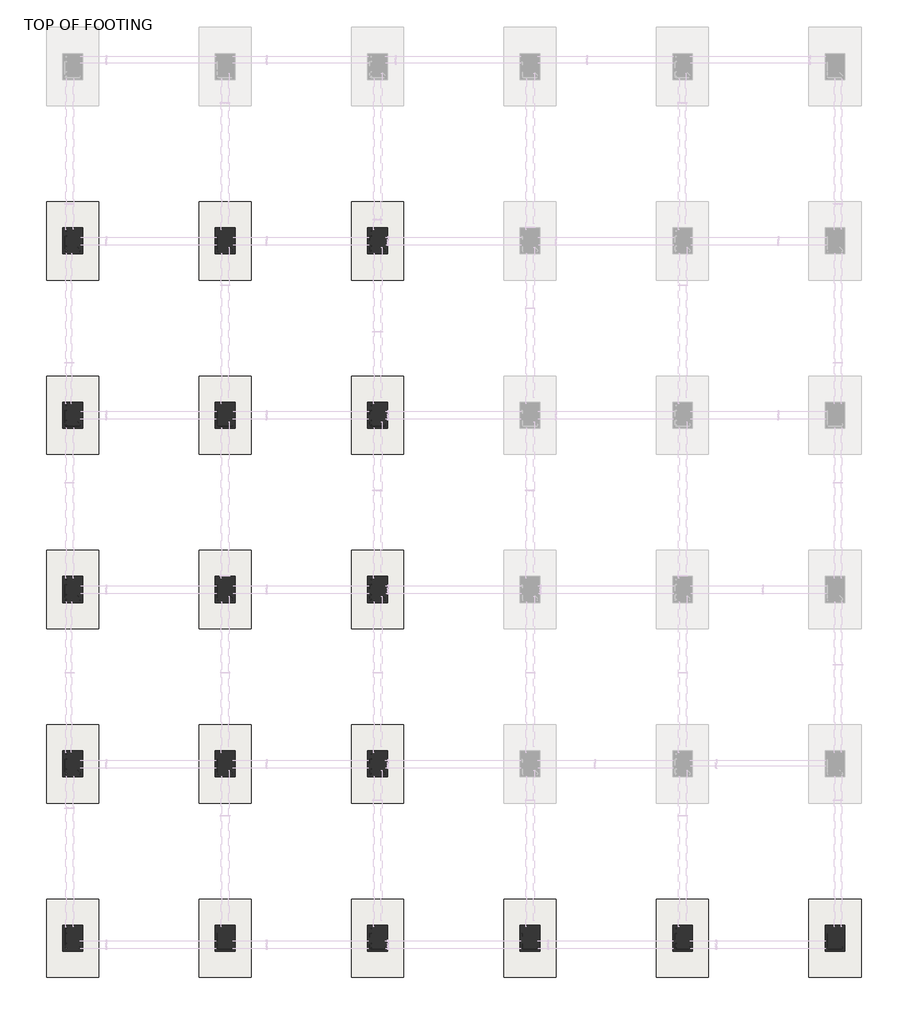
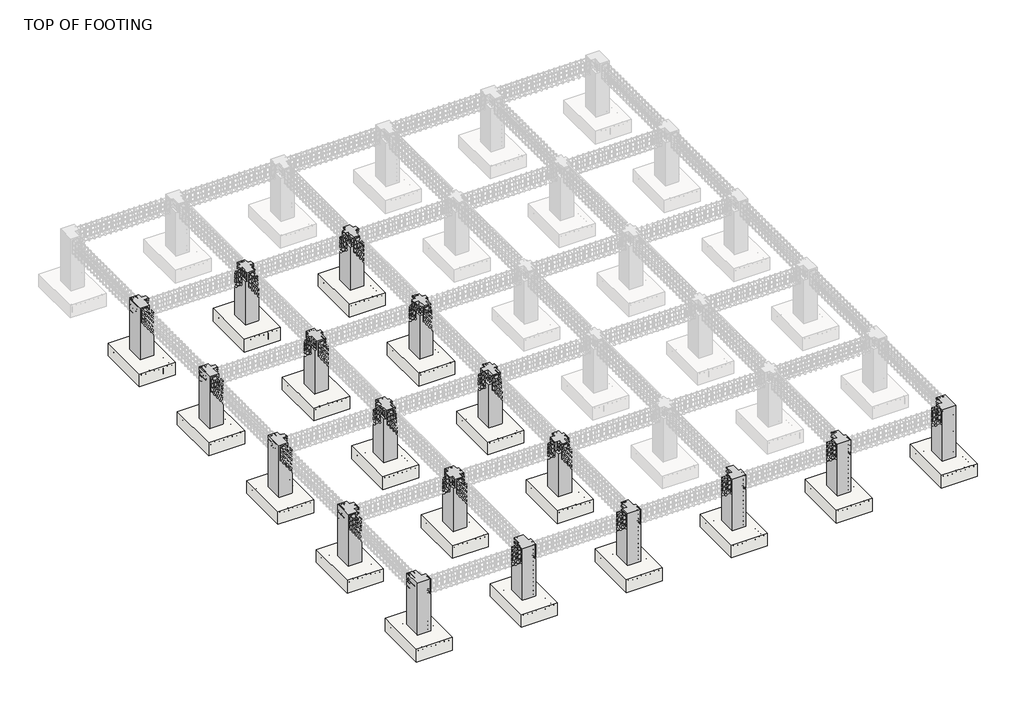
# One storey, part 1 of 33: 18 columns, 18 slabs.
"""IFC4 building model written with IfcOpenShell, lengths in millimetres."""

from ifc_helpers import new_model, si_unit, origin, place, context, project, spatial, faceted_brep, transform, mapped, element, save
from components import m_footing_rectangular_1800_x_1200_x_450mm_16ba7ea5

model = new_model("IFC4")

# Units and contexts
model_context = context("Model", 3, world=origin())
ifc_project = project(units=[si_unit("LENGTHUNIT", "METRE", prefix="MILLI")], contexts=[model_context])

# Site, building, storey
site = spatial("IfcSite", under=ifc_project)
building = spatial("IfcBuilding", under=site)
storey = spatial("IfcBuildingStorey", under=building, Name="TOP OF FOOTING", Elevation=-1828.8)

# Columns
placement = place(None, origin())
element("IfcColumn", 1, ObjectType="M_Concrete-Rectangular-Column : 450 x 600mm", at=placement, inside=storey, context=model_context, shape_type="Brep", body=[
    faceted_brep([(-8760.6788975, -214.4318674, -1828.8), (-8760.6788975, -814.4318674, -1828.8), (-9210.6788975, -814.4318674, -1828.8), (-9210.6788975, -214.4318674, -1828.8), (-8760.6788975, -214.4318674, -300.0), (-8760.6788975, -514.4318674, -300.0), (-8760.6788975, -514.4318674, 0.0), (-8760.6788975, -814.4318674, 0.0), (-9210.6788975, -814.4318674, 0.0), (-9210.6788975, -214.4318674, 0.0), (-8910.6788975, -214.4318674, 0.0), (-8910.6788975, -214.4318674, -300.0), (-8910.6788975, -514.4318674, 0.0), (-8910.6788975, -514.4318674, -300.0)], [[[0, 1, 2, 3]], [[1, 0, 4, 5, 6, 7]], [[2, 1, 7, 8]], [[3, 2, 8, 9]], [[0, 3, 9, 10, 11, 4]], [[8, 7, 6, 12, 10, 9]], [[11, 13, 5, 4]], [[13, 12, 6, 5]], [[12, 13, 11, 10]]]),
])
element("IfcColumn", 2, ObjectType="M_Concrete-Rectangular-Column : 450 x 600mm", at=placement, inside=storey, context=model_context, shape_type="Brep", body=[
    faceted_brep([(-8760.6788975, 3785.5681326, -1828.8), (-8760.6788975, 3185.5681326, -1828.8), (-9210.6788975, 3185.5681326, -1828.8), (-9210.6788975, 3785.5681326, -1828.8), (-8760.6788975, 3785.5681326, -300.0), (-8760.6788975, 3635.5681326, -300.0), (-8760.6788975, 3635.5681326, 0.0), (-8760.6788975, 3335.5681326, 0.0), (-8760.6788975, 3335.5681326, -300.0), (-8760.6788975, 3185.5681326, -300.0), (-8910.6788975, 3185.5681326, -300.0), (-8910.6788975, 3185.5681326, 0.0), (-9210.6788975, 3185.5681326, 0.0), (-9210.6788975, 3785.5681326, 0.0), (-8910.6788975, 3785.5681326, 0.0), (-8910.6788975, 3785.5681326, -300.0), (-8910.6788975, 3335.5681326, 0.0), (-8910.6788975, 3635.5681326, 0.0), (-8910.6788975, 3635.5681326, -300.0), (-8910.6788975, 3335.5681326, -300.0)], [[[0, 1, 2, 3]], [[1, 0, 4, 5, 6, 7, 8, 9]], [[2, 1, 9, 10, 11, 12]], [[3, 2, 12, 13]], [[0, 3, 13, 14, 15, 4]], [[13, 12, 11, 16, 7, 6, 17, 14]], [[15, 18, 5, 4]], [[18, 17, 6, 5]], [[17, 18, 15, 14]], [[8, 19, 10, 9]], [[19, 16, 11, 10]], [[16, 19, 8, 7]]]),
])
element("IfcColumn", 3, ObjectType="M_Concrete-Rectangular-Column : 450 x 600mm", at=placement, inside=storey, context=model_context, shape_type="Brep", body=[
    faceted_brep([(-8760.6788975, 7785.5681326, -1828.8), (-8760.6788975, 7185.5681326, -1828.8), (-9210.6788975, 7185.5681326, -1828.8), (-9210.6788975, 7785.5681326, -1828.8), (-8760.6788975, 7785.5681326, -300.0), (-8760.6788975, 7635.5681326, -300.0), (-8760.6788975, 7635.5681326, 0.0), (-8760.6788975, 7485.5681326, 0.0), (-8760.6788975, 7485.5681326, -300.0), (-8760.6788975, 7185.5681326, -300.0), (-8910.6788975, 7185.5681326, -300.0), (-8910.6788975, 7185.5681326, 0.0), (-9210.6788975, 7185.5681326, 0.0), (-9210.6788975, 7785.5681326, 0.0), (-8910.6788975, 7785.5681326, 0.0), (-8910.6788975, 7785.5681326, -300.0), (-8910.6788975, 7485.5681326, 0.0), (-8910.6788975, 7635.5681326, 0.0), (-8910.6788975, 7635.5681326, -300.0), (-8910.6788975, 7485.5681326, -300.0)], [[[0, 1, 2, 3]], [[1, 0, 4, 5, 6, 7, 8, 9]], [[2, 1, 9, 10, 11, 12]], [[3, 2, 12, 13]], [[0, 3, 13, 14, 15, 4]], [[13, 12, 11, 16, 7, 6, 17, 14]], [[15, 18, 5, 4]], [[18, 17, 6, 5]], [[17, 18, 15, 14]], [[8, 19, 10, 9]], [[19, 16, 11, 10]], [[16, 19, 8, 7]]]),
])
element("IfcColumn", 4, ObjectType="M_Concrete-Rectangular-Column : 450 x 600mm", at=placement, inside=storey, context=model_context, shape_type="Brep", body=[
    faceted_brep([(-8760.6788975, 11785.5681326, -1828.8), (-8760.6788975, 11185.5681326, -1828.8), (-9210.6788975, 11185.5681326, -1828.8), (-9210.6788975, 11785.5681326, -1828.8), (-8760.6788975, 11785.5681326, -300.0), (-8760.6788975, 11635.5681326, -300.0), (-8760.6788975, 11635.5681326, 0.0), (-8760.6788975, 11485.5681326, 0.0), (-8760.6788975, 11485.5681326, -300.0), (-8760.6788975, 11185.5681326, -300.0), (-8910.6788975, 11185.5681326, -300.0), (-8910.6788975, 11185.5681326, 0.0), (-9210.6788975, 11185.5681326, 0.0), (-9210.6788975, 11785.5681326, 0.0), (-8910.6788975, 11785.5681326, 0.0), (-8910.6788975, 11785.5681326, -300.0), (-8910.6788975, 11485.5681326, 0.0), (-8910.6788975, 11635.5681326, 0.0), (-8910.6788975, 11635.5681326, -300.0), (-8910.6788975, 11485.5681326, -300.0)], [[[0, 1, 2, 3]], [[1, 0, 4, 5, 6, 7, 8, 9]], [[2, 1, 9, 10, 11, 12]], [[3, 2, 12, 13]], [[0, 3, 13, 14, 15, 4]], [[13, 12, 11, 16, 7, 6, 17, 14]], [[15, 18, 5, 4]], [[18, 17, 6, 5]], [[17, 18, 15, 14]], [[8, 19, 10, 9]], [[19, 16, 11, 10]], [[16, 19, 8, 7]]]),
])
element("IfcColumn", 5, ObjectType="M_Concrete-Rectangular-Column : 450 x 600mm", at=placement, inside=storey, context=model_context, shape_type="Brep", body=[
    faceted_brep([(-8760.6788975, 15785.5681326, -1828.8), (-8760.6788975, 15185.5681326, -1828.8), (-9210.6788975, 15185.5681326, -1828.8), (-9210.6788975, 15785.5681326, -1828.8), (-8760.6788975, 15785.5681326, -300.0), (-8760.6788975, 15635.5681326, -300.0), (-8760.6788975, 15635.5681326, 0.0), (-8760.6788975, 15485.5681326, 0.0), (-8760.6788975, 15485.5681326, -300.0), (-8760.6788975, 15185.5681326, -300.0), (-8910.6788975, 15185.5681326, -300.0), (-8910.6788975, 15185.5681326, 0.0), (-9210.6788975, 15185.5681326, 0.0), (-9210.6788975, 15785.5681326, 0.0), (-8910.6788975, 15785.5681326, 0.0), (-8910.6788975, 15785.5681326, -300.0), (-8910.6788975, 15485.5681326, 0.0), (-8910.6788975, 15635.5681326, 0.0), (-8910.6788975, 15635.5681326, -300.0), (-8910.6788975, 15485.5681326, -300.0)], [[[0, 1, 2, 3]], [[1, 0, 4, 5, 6, 7, 8, 9]], [[2, 1, 9, 10, 11, 12]], [[3, 2, 12, 13]], [[0, 3, 13, 14, 15, 4]], [[13, 12, 11, 16, 7, 6, 17, 14]], [[15, 18, 5, 4]], [[18, 17, 6, 5]], [[17, 18, 15, 14]], [[8, 19, 10, 9]], [[19, 16, 11, 10]], [[16, 19, 8, 7]]]),
])
element("IfcColumn", 6, ObjectType="M_Concrete-Rectangular-Column : 450 x 600mm", at=placement, inside=storey, context=model_context, shape_type="Brep", body=[
    faceted_brep([(-5260.6788975, 15785.5681326, -1828.8), (-5260.6788975, 15185.5681326, -1828.8), (-5710.6788975, 15185.5681326, -1828.8), (-5710.6788975, 15785.5681326, -1828.8), (-5260.6788975, 15785.5681326, -300.0), (-5260.6788975, 15635.5681326, -300.0), (-5260.6788975, 15635.5681326, 0.0), (-5260.6788975, 15485.5681326, 0.0), (-5260.6788975, 15485.5681326, -300.0), (-5260.6788975, 15185.5681326, -300.0), (-5373.1788975, 15185.5681326, -300.0), (-5373.1788975, 15185.5681326, 0.0), (-5635.6788975, 15185.5681326, 0.0), (-5635.6788975, 15185.5681326, -300.0), (-5710.6788975, 15185.5681326, -300.0), (-5710.6788975, 15485.5681326, -300.0), (-5710.6788975, 15485.5681326, 0.0), (-5710.6788975, 15635.5681326, 0.0), (-5710.6788975, 15635.5681326, -300.0), (-5710.6788975, 15785.5681326, -300.0), (-5635.6788975, 15785.5681326, -300.0), (-5635.6788975, 15785.5681326, 0.0), (-5373.1788975, 15785.5681326, 0.0), (-5373.1788975, 15785.5681326, -300.0), (-5373.1788975, 15635.5681326, 0.0), (-5635.6788975, 15635.5681326, 0.0), (-5635.6788975, 15485.5681326, 0.0), (-5373.1788975, 15485.5681326, 0.0), (-5373.1788975, 15635.5681326, -300.0), (-5635.6788975, 15635.5681326, -300.0), (-5635.6788975, 15485.5681326, -300.0), (-5373.1788975, 15485.5681326, -300.0)], [[[0, 1, 2, 3]], [[1, 0, 4, 5, 6, 7, 8, 9]], [[2, 1, 9, 10, 11, 12, 13, 14]], [[3, 2, 14, 15, 16, 17, 18, 19]], [[0, 3, 19, 20, 21, 22, 23, 4]], [[6, 24, 22, 21, 25, 17, 16, 26, 12, 11, 27, 7]], [[23, 28, 5, 4]], [[28, 24, 6, 5]], [[24, 28, 23, 22]], [[18, 29, 20, 19]], [[29, 25, 21, 20]], [[25, 29, 18, 17]], [[30, 15, 14, 13]], [[26, 30, 13, 12]], [[30, 26, 16, 15]], [[8, 31, 10, 9]], [[31, 27, 11, 10]], [[27, 31, 8, 7]]]),
])
element("IfcColumn", 7, ObjectType="M_Concrete-Rectangular-Column : 450 x 600mm", at=placement, inside=storey, context=model_context, shape_type="Brep", body=[
    faceted_brep([(-5260.6788975, 11785.5681326, -1828.8), (-5260.6788975, 11185.5681326, -1828.8), (-5710.6788975, 11185.5681326, -1828.8), (-5710.6788975, 11785.5681326, -1828.8), (-5260.6788975, 11785.5681326, -300.0), (-5260.6788975, 11635.5681326, -300.0), (-5260.6788975, 11635.5681326, 0.0), (-5260.6788975, 11485.5681326, 0.0), (-5260.6788975, 11485.5681326, -300.0), (-5260.6788975, 11185.5681326, -300.0), (-5335.6788975, 11185.5681326, -300.0), (-5335.6788975, 11185.5681326, 0.0), (-5635.6788975, 11185.5681326, 0.0), (-5635.6788975, 11185.5681326, -300.0), (-5710.6788975, 11185.5681326, -300.0), (-5710.6788975, 11485.5681326, -300.0), (-5710.6788975, 11485.5681326, 0.0), (-5710.6788975, 11635.5681326, 0.0), (-5710.6788975, 11635.5681326, -300.0), (-5710.6788975, 11785.5681326, -300.0), (-5635.6788975, 11785.5681326, -300.0), (-5635.6788975, 11785.5681326, 0.0), (-5373.1788975, 11785.5681326, 0.0), (-5373.1788975, 11785.5681326, -300.0), (-5635.6788975, 11635.5681326, 0.0), (-5635.6788975, 11485.5681326, 0.0), (-5335.6788975, 11485.5681326, 0.0), (-5373.1788975, 11635.5681326, 0.0), (-5635.6788975, 11635.5681326, -300.0), (-5373.1788975, 11635.5681326, -300.0), (-5335.6788975, 11485.5681326, -300.0), (-5635.6788975, 11485.5681326, -300.0)], [[[0, 1, 2, 3]], [[1, 0, 4, 5, 6, 7, 8, 9]], [[2, 1, 9, 10, 11, 12, 13, 14]], [[3, 2, 14, 15, 16, 17, 18, 19]], [[0, 3, 19, 20, 21, 22, 23, 4]], [[21, 24, 17, 16, 25, 12, 11, 26, 7, 6, 27, 22]], [[18, 28, 20, 19]], [[28, 24, 21, 20]], [[24, 28, 18, 17]], [[23, 29, 5, 4]], [[29, 27, 6, 5]], [[27, 29, 23, 22]], [[8, 30, 10, 9]], [[30, 26, 11, 10]], [[26, 30, 8, 7]], [[31, 15, 14, 13]], [[25, 31, 13, 12]], [[31, 25, 16, 15]]]),
])
element("IfcColumn", 8, ObjectType="M_Concrete-Rectangular-Column : 450 x 600mm", at=placement, inside=storey, context=model_context, shape_type="Brep", body=[
    faceted_brep([(-1760.6788975, 11785.5681326, -1828.8), (-1760.6788975, 11185.5681326, -1828.8), (-2210.6788975, 11185.5681326, -1828.8), (-2210.6788975, 11785.5681326, -1828.8), (-1760.6788975, 11785.5681326, -300.0), (-1760.6788975, 11635.5681326, -300.0), (-1760.6788975, 11635.5681326, 0.0), (-1760.6788975, 11485.5681326, 0.0), (-1760.6788975, 11485.5681326, -300.0), (-1760.6788975, 11185.5681326, -300.0), (-1835.6788975, 11185.5681326, -300.0), (-1835.6788975, 11185.5681326, 0.0), (-2060.6788975, 11185.5681326, 0.0), (-2060.6788975, 11185.5681326, -300.0), (-2210.6788975, 11185.5681326, -300.0), (-2210.6788975, 11485.5681326, -300.0), (-2210.6788975, 11485.5681326, 0.0), (-2210.6788975, 11635.5681326, 0.0), (-2210.6788975, 11635.5681326, -300.0), (-2210.6788975, 11785.5681326, -300.0), (-2098.1788975, 11785.5681326, -300.0), (-2098.1788975, 11785.5681326, 0.0), (-1873.1788975, 11785.5681326, 0.0), (-1873.1788975, 11785.5681326, -300.0), (-2098.1788975, 11635.5681326, 0.0), (-2060.6788975, 11485.5681326, 0.0), (-1835.6788975, 11485.5681326, 0.0), (-1873.1788975, 11635.5681326, 0.0), (-2098.1788975, 11635.5681326, -300.0), (-1873.1788975, 11635.5681326, -300.0), (-1835.6788975, 11485.5681326, -300.0), (-2060.6788975, 11485.5681326, -300.0)], [[[0, 1, 2, 3]], [[1, 0, 4, 5, 6, 7, 8, 9]], [[2, 1, 9, 10, 11, 12, 13, 14]], [[3, 2, 14, 15, 16, 17, 18, 19]], [[0, 3, 19, 20, 21, 22, 23, 4]], [[21, 24, 17, 16, 25, 12, 11, 26, 7, 6, 27, 22]], [[18, 28, 20, 19]], [[28, 24, 21, 20]], [[24, 28, 18, 17]], [[23, 29, 5, 4]], [[29, 27, 6, 5]], [[27, 29, 23, 22]], [[8, 30, 10, 9]], [[30, 26, 11, 10]], [[26, 30, 8, 7]], [[31, 15, 14, 13]], [[25, 31, 13, 12]], [[31, 25, 16, 15]]]),
])
element("IfcColumn", 9, ObjectType="M_Concrete-Rectangular-Column : 450 x 600mm", at=placement, inside=storey, context=model_context, shape_type="Brep", body=[
    faceted_brep([(-5260.6788975, 7785.5681326, -1828.8), (-5260.6788975, 7185.5681326, -1828.8), (-5710.6788975, 7185.5681326, -1828.8), (-5710.6788975, 7785.5681326, -1828.8), (-5260.6788975, 7785.5681326, -300.0), (-5260.6788975, 7635.5681326, -300.0), (-5260.6788975, 7635.5681326, 0.0), (-5260.6788975, 7485.5681326, 0.0), (-5260.6788975, 7485.5681326, -300.0), (-5260.6788975, 7185.5681326, -300.0), (-5335.6788975, 7185.5681326, -300.0), (-5335.6788975, 7185.5681326, 0.0), (-5635.6788975, 7185.5681326, 0.0), (-5635.6788975, 7185.5681326, -300.0), (-5710.6788975, 7185.5681326, -300.0), (-5710.6788975, 7485.5681326, -300.0), (-5710.6788975, 7485.5681326, 0.0), (-5710.6788975, 7635.5681326, 0.0), (-5710.6788975, 7635.5681326, -300.0), (-5710.6788975, 7785.5681326, -300.0), (-5635.6788975, 7785.5681326, -300.0), (-5635.6788975, 7785.5681326, 0.0), (-5335.6788975, 7785.5681326, 0.0), (-5335.6788975, 7785.5681326, -300.0), (-5335.6788975, 7635.5681326, 0.0), (-5635.6788975, 7635.5681326, 0.0), (-5635.6788975, 7485.5681326, 0.0), (-5335.6788975, 7485.5681326, 0.0), (-5335.6788975, 7635.5681326, -300.0), (-5635.6788975, 7635.5681326, -300.0), (-5635.6788975, 7485.5681326, -300.0), (-5335.6788975, 7485.5681326, -300.0)], [[[0, 1, 2, 3]], [[1, 0, 4, 5, 6, 7, 8, 9]], [[2, 1, 9, 10, 11, 12, 13, 14]], [[3, 2, 14, 15, 16, 17, 18, 19]], [[0, 3, 19, 20, 21, 22, 23, 4]], [[6, 24, 22, 21, 25, 17, 16, 26, 12, 11, 27, 7]], [[23, 28, 5, 4]], [[28, 24, 6, 5]], [[24, 28, 23, 22]], [[18, 29, 20, 19]], [[29, 25, 21, 20]], [[25, 29, 18, 17]], [[30, 15, 14, 13]], [[26, 30, 13, 12]], [[30, 26, 16, 15]], [[8, 31, 10, 9]], [[31, 27, 11, 10]], [[27, 31, 8, 7]]]),
])
element("IfcColumn", 10, ObjectType="M_Concrete-Rectangular-Column : 450 x 600mm", at=placement, inside=storey, context=model_context, shape_type="Brep", body=[
    faceted_brep([(-5260.6788975, 3785.5681326, -1828.8), (-5260.6788975, 3185.5681326, -1828.8), (-5710.6788975, 3185.5681326, -1828.8), (-5710.6788975, 3785.5681326, -1828.8), (-5260.6788975, 3785.5681326, -300.0), (-5260.6788975, 3635.5681326, -300.0), (-5260.6788975, 3635.5681326, 0.0), (-5260.6788975, 3335.5681326, 0.0), (-5260.6788975, 3335.5681326, -300.0), (-5260.6788975, 3185.5681326, -300.0), (-5335.6788975, 3185.5681326, -300.0), (-5335.6788975, 3185.5681326, 0.0), (-5635.6788975, 3185.5681326, 0.0), (-5635.6788975, 3185.5681326, -300.0), (-5710.6788975, 3185.5681326, -300.0), (-5710.6788975, 3335.5681326, -300.0), (-5710.6788975, 3335.5681326, 0.0), (-5710.6788975, 3635.5681326, 0.0), (-5710.6788975, 3635.5681326, -300.0), (-5710.6788975, 3785.5681326, -300.0), (-5635.6788975, 3785.5681326, -300.0), (-5635.6788975, 3785.5681326, 0.0), (-5335.6788975, 3785.5681326, 0.0), (-5335.6788975, 3785.5681326, -300.0), (-5635.6788975, 3635.5681326, 0.0), (-5635.6788975, 3335.5681326, 0.0), (-5335.6788975, 3335.5681326, 0.0), (-5335.6788975, 3635.5681326, 0.0), (-5635.6788975, 3635.5681326, -300.0), (-5335.6788975, 3635.5681326, -300.0), (-5635.6788975, 3335.5681326, -300.0), (-5335.6788975, 3335.5681326, -300.0)], [[[0, 1, 2, 3]], [[1, 0, 4, 5, 6, 7, 8, 9]], [[2, 1, 9, 10, 11, 12, 13, 14]], [[3, 2, 14, 15, 16, 17, 18, 19]], [[0, 3, 19, 20, 21, 22, 23, 4]], [[21, 24, 17, 16, 25, 12, 11, 26, 7, 6, 27, 22]], [[18, 28, 20, 19]], [[28, 24, 21, 20]], [[24, 28, 18, 17]], [[23, 29, 5, 4]], [[29, 27, 6, 5]], [[27, 29, 23, 22]], [[30, 15, 14, 13]], [[25, 30, 13, 12]], [[30, 25, 16, 15]], [[8, 31, 10, 9]], [[31, 26, 11, 10]], [[26, 31, 8, 7]]]),
])
element("IfcColumn", 11, ObjectType="M_Concrete-Rectangular-Column : 450 x 600mm", at=placement, inside=storey, context=model_context, shape_type="Brep", body=[
    faceted_brep([(-5260.6788975, -214.4318674, -1828.8), (-5260.6788975, -814.4318674, -1828.8), (-5710.6788975, -814.4318674, -1828.8), (-5710.6788975, -214.4318674, -1828.8), (-5260.6788975, -214.4318674, -300.0), (-5260.6788975, -514.4318674, -300.0), (-5260.6788975, -514.4318674, 0.0), (-5260.6788975, -814.4318674, 0.0), (-5710.6788975, -814.4318674, 0.0), (-5710.6788975, -514.4318674, 0.0), (-5710.6788975, -514.4318674, -300.0), (-5710.6788975, -214.4318674, -300.0), (-5635.6788975, -214.4318674, -300.0), (-5635.6788975, -214.4318674, 0.0), (-5335.6788975, -214.4318674, 0.0), (-5335.6788975, -214.4318674, -300.0), (-5335.6788975, -514.4318674, 0.0), (-5635.6788975, -514.4318674, 0.0), (-5635.6788975, -514.4318674, -300.0), (-5335.6788975, -514.4318674, -300.0)], [[[0, 1, 2, 3]], [[1, 0, 4, 5, 6, 7]], [[2, 1, 7, 8]], [[3, 2, 8, 9, 10, 11]], [[0, 3, 11, 12, 13, 14, 15, 4]], [[8, 7, 6, 16, 14, 13, 17, 9]], [[10, 18, 12, 11]], [[18, 17, 13, 12]], [[17, 18, 10, 9]], [[15, 19, 5, 4]], [[19, 16, 6, 5]], [[16, 19, 15, 14]]]),
])
element("IfcColumn", 12, ObjectType="M_Concrete-Rectangular-Column : 450 x 600mm", at=placement, inside=storey, context=model_context, shape_type="Brep", body=[
    faceted_brep([(-1760.6788975, -214.4318674, -1828.8), (-1760.6788975, -814.4318674, -1828.8), (-2210.6788975, -814.4318674, -1828.8), (-2210.6788975, -214.4318674, -1828.8), (-1760.6788975, -214.4318674, -300.0), (-1760.6788975, -514.4318674, -300.0), (-1760.6788975, -514.4318674, 0.0), (-1760.6788975, -814.4318674, 0.0), (-2210.6788975, -814.4318674, 0.0), (-2210.6788975, -514.4318674, 0.0), (-2210.6788975, -514.4318674, -300.0), (-2210.6788975, -214.4318674, -300.0), (-2060.6788975, -214.4318674, -300.0), (-2060.6788975, -214.4318674, 0.0), (-1835.6788975, -214.4318674, 0.0), (-1835.6788975, -214.4318674, -300.0), (-1835.6788975, -514.4318674, 0.0), (-2060.6788975, -514.4318674, 0.0), (-2060.6788975, -514.4318674, -300.0), (-1835.6788975, -514.4318674, -300.0)], [[[0, 1, 2, 3]], [[1, 0, 4, 5, 6, 7]], [[2, 1, 7, 8]], [[3, 2, 8, 9, 10, 11]], [[0, 3, 11, 12, 13, 14, 15, 4]], [[8, 7, 6, 16, 14, 13, 17, 9]], [[10, 18, 12, 11]], [[18, 17, 13, 12]], [[17, 18, 10, 9]], [[15, 19, 5, 4]], [[19, 16, 6, 5]], [[16, 19, 15, 14]]]),
])
element("IfcColumn", 13, ObjectType="M_Concrete-Rectangular-Column : 450 x 600mm", at=placement, inside=storey, context=model_context, shape_type="Brep", body=[
    faceted_brep([(-1760.6788975, 3785.5681326, -1828.8), (-1760.6788975, 3185.5681326, -1828.8), (-2210.6788975, 3185.5681326, -1828.8), (-2210.6788975, 3785.5681326, -1828.8), (-1760.6788975, 3785.5681326, -300.0), (-1760.6788975, 3635.5681326, -300.0), (-1760.6788975, 3635.5681326, 0.0), (-1760.6788975, 3335.5681326, 0.0), (-1760.6788975, 3335.5681326, -300.0), (-1760.6788975, 3185.5681326, -300.0), (-1835.6788975, 3185.5681326, -300.0), (-1835.6788975, 3185.5681326, 0.0), (-2060.6788975, 3185.5681326, 0.0), (-2060.6788975, 3185.5681326, -300.0), (-2210.6788975, 3185.5681326, -300.0), (-2210.6788975, 3335.5681326, -300.0), (-2210.6788975, 3335.5681326, 0.0), (-2210.6788975, 3635.5681326, 0.0), (-2210.6788975, 3635.5681326, -300.0), (-2210.6788975, 3785.5681326, -300.0), (-2060.6788975, 3785.5681326, -300.0), (-2060.6788975, 3785.5681326, 0.0), (-1835.6788975, 3785.5681326, 0.0), (-1835.6788975, 3785.5681326, -300.0), (-2060.6788975, 3635.5681326, 0.0), (-2060.6788975, 3335.5681326, 0.0), (-1835.6788975, 3335.5681326, 0.0), (-1835.6788975, 3635.5681326, 0.0), (-2060.6788975, 3635.5681326, -300.0), (-1835.6788975, 3635.5681326, -300.0), (-2060.6788975, 3335.5681326, -300.0), (-1835.6788975, 3335.5681326, -300.0)], [[[0, 1, 2, 3]], [[1, 0, 4, 5, 6, 7, 8, 9]], [[2, 1, 9, 10, 11, 12, 13, 14]], [[3, 2, 14, 15, 16, 17, 18, 19]], [[0, 3, 19, 20, 21, 22, 23, 4]], [[21, 24, 17, 16, 25, 12, 11, 26, 7, 6, 27, 22]], [[18, 28, 20, 19]], [[28, 24, 21, 20]], [[24, 28, 18, 17]], [[23, 29, 5, 4]], [[29, 27, 6, 5]], [[27, 29, 23, 22]], [[30, 15, 14, 13]], [[25, 30, 13, 12]], [[30, 25, 16, 15]], [[8, 31, 10, 9]], [[31, 26, 11, 10]], [[26, 31, 8, 7]]]),
])
element("IfcColumn", 14, ObjectType="M_Concrete-Rectangular-Column : 450 x 600mm", at=placement, inside=storey, context=model_context, shape_type="Brep", body=[
    faceted_brep([(-1760.6788975, 7785.5681326, -1828.8), (-1760.6788975, 7185.5681326, -1828.8), (-2210.6788975, 7185.5681326, -1828.8), (-2210.6788975, 7785.5681326, -1828.8), (-1760.6788975, 7785.5681326, -300.0), (-1760.6788975, 7635.5681326, -300.0), (-1760.6788975, 7635.5681326, 0.0), (-1760.6788975, 7485.5681326, 0.0), (-1760.6788975, 7485.5681326, -300.0), (-1760.6788975, 7185.5681326, -300.0), (-1835.6788975, 7185.5681326, -300.0), (-1835.6788975, 7185.5681326, 0.0), (-2060.6788975, 7185.5681326, 0.0), (-2060.6788975, 7185.5681326, -300.0), (-2210.6788975, 7185.5681326, -300.0), (-2210.6788975, 7485.5681326, -300.0), (-2210.6788975, 7485.5681326, 0.0), (-2210.6788975, 7635.5681326, 0.0), (-2210.6788975, 7635.5681326, -300.0), (-2210.6788975, 7785.5681326, -300.0), (-2060.6788975, 7785.5681326, -300.0), (-2060.6788975, 7785.5681326, 0.0), (-1835.6788975, 7785.5681326, 0.0), (-1835.6788975, 7785.5681326, -300.0), (-1835.6788975, 7635.5681326, 0.0), (-2060.6788975, 7635.5681326, 0.0), (-2060.6788975, 7485.5681326, 0.0), (-1835.6788975, 7485.5681326, 0.0), (-1835.6788975, 7635.5681326, -300.0), (-2060.6788975, 7635.5681326, -300.0), (-2060.6788975, 7485.5681326, -300.0), (-1835.6788975, 7485.5681326, -300.0)], [[[0, 1, 2, 3]], [[1, 0, 4, 5, 6, 7, 8, 9]], [[2, 1, 9, 10, 11, 12, 13, 14]], [[3, 2, 14, 15, 16, 17, 18, 19]], [[0, 3, 19, 20, 21, 22, 23, 4]], [[6, 24, 22, 21, 25, 17, 16, 26, 12, 11, 27, 7]], [[23, 28, 5, 4]], [[28, 24, 6, 5]], [[24, 28, 23, 22]], [[18, 29, 20, 19]], [[29, 25, 21, 20]], [[25, 29, 18, 17]], [[30, 15, 14, 13]], [[26, 30, 13, 12]], [[30, 26, 16, 15]], [[8, 31, 10, 9]], [[31, 27, 11, 10]], [[27, 31, 8, 7]]]),
])
element("IfcColumn", 15, ObjectType="M_Concrete-Rectangular-Column : 450 x 600mm", at=placement, inside=storey, context=model_context, shape_type="Brep", body=[
    faceted_brep([(-1760.6788975, 15785.5681326, -1828.8), (-1760.6788975, 15185.5681326, -1828.8), (-2210.6788975, 15185.5681326, -1828.8), (-2210.6788975, 15785.5681326, -1828.8), (-1760.6788975, 15785.5681326, -300.0), (-1760.6788975, 15635.5681326, -300.0), (-1760.6788975, 15635.5681326, 0.0), (-1760.6788975, 15485.5681326, 0.0), (-1760.6788975, 15485.5681326, -300.0), (-1760.6788975, 15185.5681326, -300.0), (-1873.1788975, 15185.5681326, -300.0), (-1873.1788975, 15185.5681326, 0.0), (-2098.1788975, 15185.5681326, 0.0), (-2098.1788975, 15185.5681326, -300.0), (-2210.6788975, 15185.5681326, -300.0), (-2210.6788975, 15485.5681326, -300.0), (-2210.6788975, 15485.5681326, 0.0), (-2210.6788975, 15635.5681326, 0.0), (-2210.6788975, 15635.5681326, -300.0), (-2210.6788975, 15785.5681326, -300.0), (-2098.1788975, 15785.5681326, -300.0), (-2098.1788975, 15785.5681326, 0.0), (-1873.1788975, 15785.5681326, 0.0), (-1873.1788975, 15785.5681326, -300.0), (-1873.1788975, 15635.5681326, 0.0), (-2098.1788975, 15635.5681326, 0.0), (-2098.1788975, 15485.5681326, 0.0), (-1873.1788975, 15485.5681326, 0.0), (-1873.1788975, 15635.5681326, -300.0), (-2098.1788975, 15635.5681326, -300.0), (-2098.1788975, 15485.5681326, -300.0), (-1873.1788975, 15485.5681326, -300.0)], [[[0, 1, 2, 3]], [[1, 0, 4, 5, 6, 7, 8, 9]], [[2, 1, 9, 10, 11, 12, 13, 14]], [[3, 2, 14, 15, 16, 17, 18, 19]], [[0, 3, 19, 20, 21, 22, 23, 4]], [[6, 24, 22, 21, 25, 17, 16, 26, 12, 11, 27, 7]], [[23, 28, 5, 4]], [[28, 24, 6, 5]], [[24, 28, 23, 22]], [[18, 29, 20, 19]], [[29, 25, 21, 20]], [[25, 29, 18, 17]], [[30, 15, 14, 13]], [[26, 30, 13, 12]], [[30, 26, 16, 15]], [[8, 31, 10, 9]], [[31, 27, 11, 10]], [[27, 31, 8, 7]]]),
])
element("IfcColumn", 16, ObjectType="M_Concrete-Rectangular-Column : 450 x 600mm", at=placement, inside=storey, context=model_context, shape_type="Brep", body=[
    faceted_brep([(1739.3211025, -214.4318674, -1828.8), (1739.3211025, -814.4318674, -1828.8), (1289.3211025, -814.4318674, -1828.8), (1289.3211025, -214.4318674, -1828.8), (1739.3211025, -214.4318674, -300.0), (1739.3211025, -514.4318674, -300.0), (1739.3211025, -514.4318674, 0.0), (1739.3211025, -814.4318674, 0.0), (1289.3211025, -814.4318674, 0.0), (1289.3211025, -514.4318674, 0.0), (1289.3211025, -514.4318674, -300.0), (1289.3211025, -214.4318674, -300.0), (1439.3211025, -214.4318674, -300.0), (1439.3211025, -214.4318674, 0.0), (1664.3211025, -214.4318674, 0.0), (1664.3211025, -214.4318674, -300.0), (1664.3211025, -514.4318674, 0.0), (1439.3211025, -514.4318674, 0.0), (1439.3211025, -514.4318674, -300.0), (1664.3211025, -514.4318674, -300.0)], [[[0, 1, 2, 3]], [[1, 0, 4, 5, 6, 7]], [[2, 1, 7, 8]], [[3, 2, 8, 9, 10, 11]], [[0, 3, 11, 12, 13, 14, 15, 4]], [[8, 7, 6, 16, 14, 13, 17, 9]], [[10, 18, 12, 11]], [[18, 17, 13, 12]], [[17, 18, 10, 9]], [[15, 19, 5, 4]], [[19, 16, 6, 5]], [[16, 19, 15, 14]]]),
])
element("IfcColumn", 17, ObjectType="M_Concrete-Rectangular-Column : 450 x 600mm", at=placement, inside=storey, context=model_context, shape_type="Brep", body=[
    faceted_brep([(5239.3211025, -214.4318674, -1828.8), (5239.3211025, -814.4318674, -1828.8), (4789.3211025, -814.4318674, -1828.8), (4789.3211025, -214.4318674, -1828.8), (5239.3211025, -214.4318674, -300.0), (5239.3211025, -514.4318674, -300.0), (5239.3211025, -514.4318674, 0.0), (5239.3211025, -814.4318674, 0.0), (4789.3211025, -814.4318674, 0.0), (4789.3211025, -514.4318674, 0.0), (4789.3211025, -514.4318674, -300.0), (4789.3211025, -214.4318674, -300.0), (4939.3211025, -214.4318674, -300.0), (4939.3211025, -214.4318674, 0.0), (5164.3211025, -214.4318674, 0.0), (5164.3211025, -214.4318674, -300.0), (5164.3211025, -514.4318674, 0.0), (4939.3211025, -514.4318674, 0.0), (4939.3211025, -514.4318674, -300.0), (5164.3211025, -514.4318674, -300.0)], [[[0, 1, 2, 3]], [[1, 0, 4, 5, 6, 7]], [[2, 1, 7, 8]], [[3, 2, 8, 9, 10, 11]], [[0, 3, 11, 12, 13, 14, 15, 4]], [[8, 7, 6, 16, 14, 13, 17, 9]], [[10, 18, 12, 11]], [[18, 17, 13, 12]], [[17, 18, 10, 9]], [[15, 19, 5, 4]], [[19, 16, 6, 5]], [[16, 19, 15, 14]]]),
])
element("IfcColumn", 18, ObjectType="M_Concrete-Rectangular-Column : 450 x 600mm", at=placement, inside=storey, context=model_context, shape_type="Brep", body=[
    faceted_brep([(8739.3211025, -214.4318674, -1828.8), (8739.3211025, -814.4318674, -1828.8), (8289.3211025, -814.4318674, -1828.8), (8289.3211025, -214.4318674, -1828.8), (8739.3211025, -214.4318674, 0.0), (8739.3211025, -814.4318674, 0.0), (8289.3211025, -814.4318674, 0.0), (8289.3211025, -514.4318674, 0.0), (8289.3211025, -514.4318674, -300.0), (8289.3211025, -214.4318674, -300.0), (8439.3211025, -214.4318674, -300.0), (8439.3211025, -214.4318674, 0.0), (8439.3211025, -514.4318674, 0.0), (8439.3211025, -514.4318674, -300.0)], [[[0, 1, 2, 3]], [[1, 0, 4, 5]], [[2, 1, 5, 6]], [[3, 2, 6, 7, 8, 9]], [[0, 3, 9, 10, 11, 4]], [[5, 4, 11, 12, 7, 6]], [[8, 13, 10, 9]], [[13, 12, 11, 10]], [[12, 13, 8, 7]]]),
])

# Slabs
m_footing_rectangular_1800_x_1200_x_450mm_shape = m_footing_rectangular_1800_x_1200_x_450mm_16ba7ea5(model_context)
element("IfcSlab", 19, ObjectType="M_Footing-Rectangular : 1800 x 1200 x 450mm", at=placement, inside=storey, context=model_context, shape_type="MappedRepresentation", body=[
    mapped(m_footing_rectangular_1800_x_1200_x_450mm_shape, transform((-8985.6788975, 15485.5681326, -1828.8), x_axis=(1.0, 0.0, 0.0), y_axis=(0.0, 1.0, 0.0), z_axis=(0.0, 0.0, 1.0))),
])
element("IfcSlab", 20, ObjectType="M_Footing-Rectangular : 1800 x 1200 x 450mm", at=placement, inside=storey, context=model_context, shape_type="MappedRepresentation", body=[
    mapped(m_footing_rectangular_1800_x_1200_x_450mm_shape, transform((-8985.6788975, 11485.5681326, -1828.8), x_axis=(1.0, 0.0, 0.0), y_axis=(0.0, 1.0, 0.0), z_axis=(0.0, 0.0, 1.0))),
])
element("IfcSlab", 21, ObjectType="M_Footing-Rectangular : 1800 x 1200 x 450mm", at=placement, inside=storey, context=model_context, shape_type="MappedRepresentation", body=[
    mapped(m_footing_rectangular_1800_x_1200_x_450mm_shape, transform((-8985.6788975, 7485.5681326, -1828.8), x_axis=(1.0, 0.0, 0.0), y_axis=(0.0, 1.0, 0.0), z_axis=(0.0, 0.0, 1.0))),
])
element("IfcSlab", 22, ObjectType="M_Footing-Rectangular : 1800 x 1200 x 450mm", at=placement, inside=storey, context=model_context, shape_type="MappedRepresentation", body=[
    mapped(m_footing_rectangular_1800_x_1200_x_450mm_shape, transform((-8985.6788975, 3485.5681326, -1828.8), x_axis=(1.0, 0.0, 0.0), y_axis=(0.0, 1.0, 0.0), z_axis=(0.0, 0.0, 1.0))),
])
element("IfcSlab", 23, ObjectType="M_Footing-Rectangular : 1800 x 1200 x 450mm", at=placement, inside=storey, context=model_context, shape_type="MappedRepresentation", body=[
    mapped(m_footing_rectangular_1800_x_1200_x_450mm_shape, transform((-8985.6788975, -514.4318674, -1828.8), x_axis=(1.0, 0.0, 0.0), y_axis=(0.0, 1.0, 0.0), z_axis=(0.0, 0.0, 1.0))),
])
element("IfcSlab", 24, ObjectType="M_Footing-Rectangular : 1800 x 1200 x 450mm", at=placement, inside=storey, context=model_context, shape_type="MappedRepresentation", body=[
    mapped(m_footing_rectangular_1800_x_1200_x_450mm_shape, transform((-5485.6788975, 15485.5681326, -1828.8), x_axis=(1.0, 0.0, 0.0), y_axis=(0.0, 1.0, 0.0), z_axis=(0.0, 0.0, 1.0))),
])
element("IfcSlab", 25, ObjectType="M_Footing-Rectangular : 1800 x 1200 x 450mm", at=placement, inside=storey, context=model_context, shape_type="MappedRepresentation", body=[
    mapped(m_footing_rectangular_1800_x_1200_x_450mm_shape, transform((-5485.6788975, 11485.5681326, -1828.8), x_axis=(1.0, 0.0, 0.0), y_axis=(0.0, 1.0, 0.0), z_axis=(0.0, 0.0, 1.0))),
])
element("IfcSlab", 26, ObjectType="M_Footing-Rectangular : 1800 x 1200 x 450mm", at=placement, inside=storey, context=model_context, shape_type="MappedRepresentation", body=[
    mapped(m_footing_rectangular_1800_x_1200_x_450mm_shape, transform((-5485.6788975, 7485.5681326, -1828.8), x_axis=(1.0, 0.0, 0.0), y_axis=(0.0, 1.0, 0.0), z_axis=(0.0, 0.0, 1.0))),
])
element("IfcSlab", 27, ObjectType="M_Footing-Rectangular : 1800 x 1200 x 450mm", at=placement, inside=storey, context=model_context, shape_type="MappedRepresentation", body=[
    mapped(m_footing_rectangular_1800_x_1200_x_450mm_shape, transform((-5485.6788975, 3485.5681326, -1828.8), x_axis=(1.0, 0.0, 0.0), y_axis=(0.0, 1.0, 0.0), z_axis=(0.0, 0.0, 1.0))),
])
element("IfcSlab", 28, ObjectType="M_Footing-Rectangular : 1800 x 1200 x 450mm", at=placement, inside=storey, context=model_context, shape_type="MappedRepresentation", body=[
    mapped(m_footing_rectangular_1800_x_1200_x_450mm_shape, transform((-5485.6788975, -514.4318674, -1828.8), x_axis=(1.0, 0.0, 0.0), y_axis=(0.0, 1.0, 0.0), z_axis=(0.0, 0.0, 1.0))),
])
element("IfcSlab", 29, ObjectType="M_Footing-Rectangular : 1800 x 1200 x 450mm", at=placement, inside=storey, context=model_context, shape_type="MappedRepresentation", body=[
    mapped(m_footing_rectangular_1800_x_1200_x_450mm_shape, transform((-1985.6788975, 15485.5681326, -1828.8), x_axis=(1.0, 0.0, 0.0), y_axis=(0.0, 1.0, 0.0), z_axis=(0.0, 0.0, 1.0))),
])
element("IfcSlab", 30, ObjectType="M_Footing-Rectangular : 1800 x 1200 x 450mm", at=placement, inside=storey, context=model_context, shape_type="MappedRepresentation", body=[
    mapped(m_footing_rectangular_1800_x_1200_x_450mm_shape, transform((-1985.6788975, 11485.5681326, -1828.8), x_axis=(1.0, 0.0, 0.0), y_axis=(0.0, 1.0, 0.0), z_axis=(0.0, 0.0, 1.0))),
])
element("IfcSlab", 31, ObjectType="M_Footing-Rectangular : 1800 x 1200 x 450mm", at=placement, inside=storey, context=model_context, shape_type="MappedRepresentation", body=[
    mapped(m_footing_rectangular_1800_x_1200_x_450mm_shape, transform((-1985.6788975, 7485.5681326, -1828.8), x_axis=(1.0, 0.0, 0.0), y_axis=(0.0, 1.0, 0.0), z_axis=(0.0, 0.0, 1.0))),
])
element("IfcSlab", 32, ObjectType="M_Footing-Rectangular : 1800 x 1200 x 450mm", at=placement, inside=storey, context=model_context, shape_type="MappedRepresentation", body=[
    mapped(m_footing_rectangular_1800_x_1200_x_450mm_shape, transform((-1985.6788975, 3485.5681326, -1828.8), x_axis=(1.0, 0.0, 0.0), y_axis=(0.0, 1.0, 0.0), z_axis=(0.0, 0.0, 1.0))),
])
element("IfcSlab", 33, ObjectType="M_Footing-Rectangular : 1800 x 1200 x 450mm", at=placement, inside=storey, context=model_context, shape_type="MappedRepresentation", body=[
    mapped(m_footing_rectangular_1800_x_1200_x_450mm_shape, transform((-1985.6788975, -514.4318674, -1828.8), x_axis=(1.0, 0.0, 0.0), y_axis=(0.0, 1.0, 0.0), z_axis=(0.0, 0.0, 1.0))),
])
element("IfcSlab", 34, ObjectType="M_Footing-Rectangular : 1800 x 1200 x 450mm", at=placement, inside=storey, context=model_context, shape_type="MappedRepresentation", body=[
    mapped(m_footing_rectangular_1800_x_1200_x_450mm_shape, transform((1514.3211025, -514.4318674, -1828.8), x_axis=(1.0, 0.0, 0.0), y_axis=(0.0, 1.0, 0.0), z_axis=(0.0, 0.0, 1.0))),
])
element("IfcSlab", 35, ObjectType="M_Footing-Rectangular : 1800 x 1200 x 450mm", at=placement, inside=storey, context=model_context, shape_type="MappedRepresentation", body=[
    mapped(m_footing_rectangular_1800_x_1200_x_450mm_shape, transform((5014.3211025, -514.4318674, -1828.8), x_axis=(1.0, 0.0, 0.0), y_axis=(0.0, 1.0, 0.0), z_axis=(0.0, 0.0, 1.0))),
])
element("IfcSlab", 36, ObjectType="M_Footing-Rectangular : 1800 x 1200 x 450mm", at=placement, inside=storey, context=model_context, shape_type="MappedRepresentation", body=[
    mapped(m_footing_rectangular_1800_x_1200_x_450mm_shape, transform((8514.3211025, -514.4318674, -1828.8), x_axis=(1.0, 0.0, 0.0), y_axis=(0.0, 1.0, 0.0), z_axis=(0.0, 0.0, 1.0))),
])

save(model, "model.ifc")

# Revit data of these elements
# Grids (mm)
#   "1": line (-8985.679, 28768.468) -> (-8985.679, -13113.61)
#   "2": line (-5485.679, 28768.468) -> (-5485.679, -13113.61)
#   "3": line (-1985.679, 28768.468) -> (-1985.679, -13113.61)
#   "4": line (1514.321, 28768.468) -> (1514.321, -13113.61)
#   "5": line (5014.321, 28768.468) -> (5014.321, -13113.61)
#   "6": line (8514.321, 28768.468) -> (8514.321, -13113.61)
#   "A": line (18066.759, 19485.568) -> (-10153.413, 19485.568)
#   "B": line (18066.759, 15485.568) -> (-10153.413, 15485.568)
#   "C": line (18066.759, 11485.568) -> (-10153.413, 11485.568)
#   "D": line (18066.759, 7485.568) -> (-10153.413, 7485.568)
#   "E": line (18066.759, 3485.568) -> (-10153.413, 3485.568)
#   "F": line (18066.759, -514.432) -> (-10153.413, -514.432)
# Type "M_Concrete-Rectangular-Column : 450 x 600mm"
#   b = 450 mm
#   h = 600 mm
#   Structural Material [instance default] = Concrete, Cast-in-Place gray
# Type "M_Footing-Rectangular : 1800 x 1200 x 450mm"
#   Width = 1200 mm
#   Length = 1800 mm
#   Foundation Thickness = 450 mm
#   Structural Material [instance default] = Concrete, Cast-in-Place gray
#   Assembly Code = ""
# Elements 1, 2, 3, 4, 5, 6, 7, 8, 9, 10, 11, 12, 13, 14, 15, 16, 17, 18 (IfcColumn, "M_Concrete-Rectangular-Column : 450 x 600mm")
#   Structural Material = Concrete, Cast-in-Place gray
#   Phase Created = New Construction
#   Materials on its faces: "Concrete, Cast-in-Place gray"
# Elements 19, 20, 21, 22, 23, 24, 25, 26, 27, 28, 29, 30, 31, 32, 33, 34, 35, 36 (IfcSlab, "M_Footing-Rectangular : 1800 x 1200 x 450mm")
#   Structural Material = Concrete, Cast-in-Place gray
#   Phase Created = New Construction
#   Materials on its faces: "Concrete, Cast-in-Place gray"
# Materials
#   "Concrete, Cast-in-Place gray": class "Concrete", colour RGB 192 192 192, transparency 0, Description = "Cast-in-place concrete", Cost = 0
